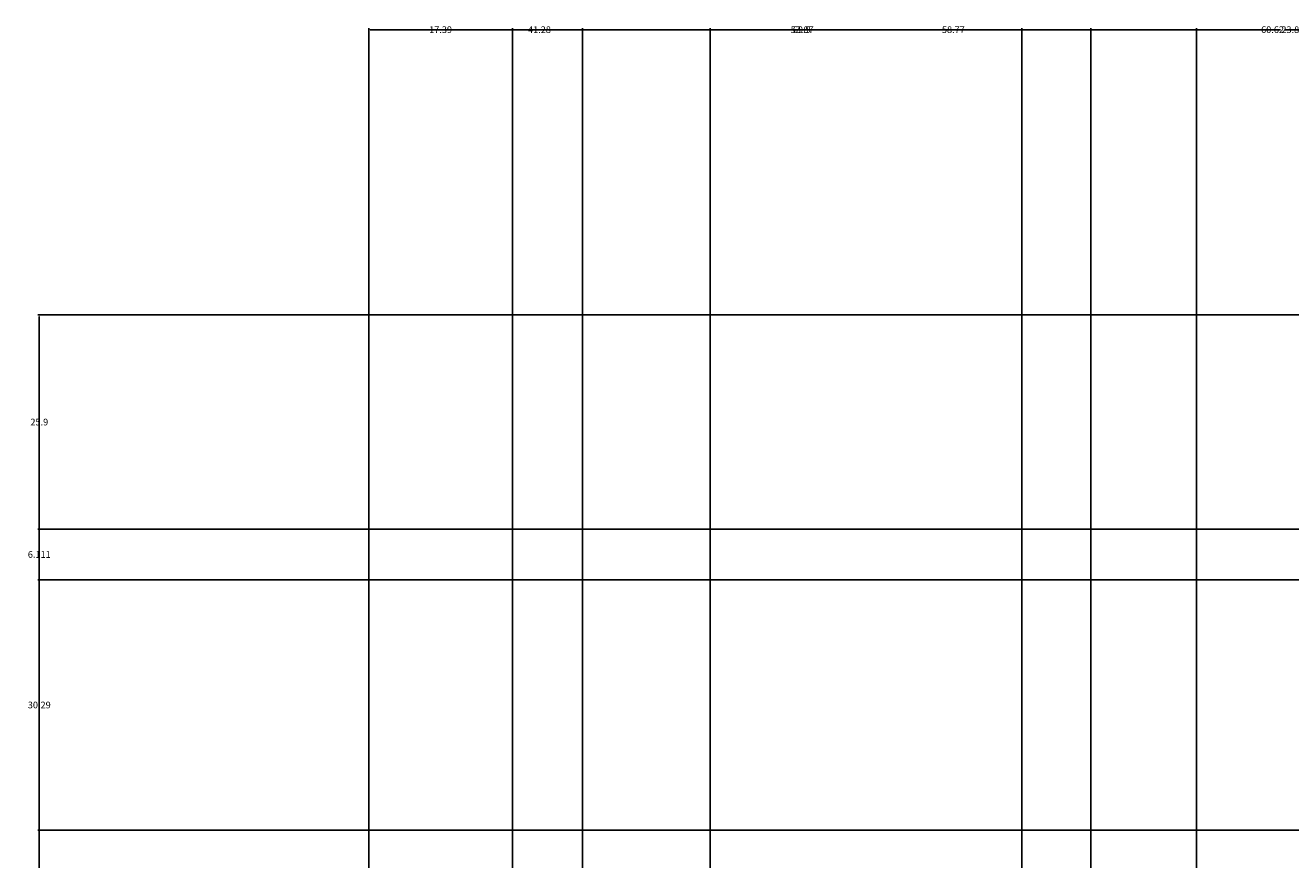
# Model space of a CAD drawing. Units: inches. Extents: x 36 to 594, y 79 to 831.
# Tile 22 of 30: x 36 to 189, y 730 to 831. Entities that reach past the tile are written whole.
import ezdxf

# ---------------------------------------------------------------- set-up
doc = ezdxf.new("R2010")
doc.units = ezdxf.units.IN
doc.header["$MEASUREMENT"] = 0
doc.layers.add('A-ANNO-DIMS', color=2, linetype='Continuous', lineweight=18)
doc.styles.get("Standard").update_dxf_attribs({"font": 'arial.ttf'})
doc.dimstyles.get("Standard").update_dxf_attribs({"dimtxt": 0.8125, "dimasz": 0.18, "dimexe": 0.18, "dimexo": 0.0625, "dimgap": 0.09, "dimtad": 0, "dimtih": 1, "dimtoh": 1, "dimdec": 4, "dimzin": 0, "dimdsep": 46, "dimlunit": 4, "dimtxsty": 'Standard', "dimcen": 0.09, "dimadec": 0, "dimazin": 0, "dimtfac": 1, "dimtdec": 4, "dimtofl": 0, "dimtmove": 0, "dimatfit": 3, "dimfxl": 1, "dimtolj": 1, "dimtzin": 0, "dimarcsym": 0})

# ---------------------------------------------------------------- blocks, each defined once
blk = doc.blocks.new('*D12')
at = {"layer": 'A-ANNO-DIMS', "color": 0, "lineweight": -2, "transparency": 16777216}
for p, q in [((77.48, 667.8), (77.48, 830.73)), ((77.66, 830.55), (96.64, 830.55)), ((118.58, 830.55), (99.6, 830.55)), ((118.76, 594.27), (118.76, 830.73))]:
    blk.add_line(p, q, dxfattribs=at)
at = {"layer": 'A-ANNO-DIMS', "color": 0, "transparency": 16777216}
for points in [[(77.66, 830.58), (77.66, 830.52), (77.48, 830.55)], [(118.58, 830.58), (118.58, 830.52), (118.76, 830.55)]]:
    blk.add_solid(points, dxfattribs=at)
at = {"layer": 'Defpoints', "color": 0, "transparency": 16777216}
for p in [(118.76, 830.55), (77.48, 667.73), (118.76, 594.21)]:
    blk.add_point(p, dxfattribs=at)
at = {"layer": 'A-ANNO-DIMS', "color": 0, "transparency": 16777216, "insert": (98.12, 830.55), "char_height": 0.812, "attachment_point": 5}
blk.add_mtext('\\A1;41.28', dxfattribs=at)
blk = doc.blocks.new('*D13')
at = {"layer": 'A-ANNO-DIMS', "color": 0, "lineweight": -2, "transparency": 16777216}
for p, q in [((118.76, 594.27), (118.76, 830.73)), ((118.94, 830.55), (146.68, 830.55)), ((177.34, 830.55), (149.6, 830.55)), ((177.52, 594.27), (177.52, 830.73))]:
    blk.add_line(p, q, dxfattribs=at)
at = {"layer": 'A-ANNO-DIMS', "color": 0, "transparency": 16777216}
for points in [[(118.94, 830.58), (118.94, 830.52), (118.76, 830.55)], [(177.34, 830.58), (177.34, 830.52), (177.52, 830.55)]]:
    blk.add_solid(points, dxfattribs=at)
at = {"layer": 'Defpoints', "color": 0, "transparency": 16777216}
for p in [(177.52, 830.55), (118.76, 594.21), (177.52, 594.21)]:
    blk.add_point(p, dxfattribs=at)
at = {"layer": 'A-ANNO-DIMS', "color": 0, "transparency": 16777216, "insert": (148.14, 830.55), "char_height": 0.812, "attachment_point": 5}
blk.add_mtext('\\A1;58.77', dxfattribs=at)
blk = doc.blocks.new('*D14')
at = {"layer": 'A-ANNO-DIMS', "color": 0, "lineweight": -2, "transparency": 16777216}
for p, q in [((177.52, 594.27), (177.52, 830.73)), ((177.7, 830.55), (187.69, 830.55)), ((201.24, 830.55), (191.25, 830.55)), ((201.42, 720.66), (201.42, 830.73))]:
    blk.add_line(p, q, dxfattribs=at)
at = {"layer": 'A-ANNO-DIMS', "color": 0, "transparency": 16777216}
for points in [[(177.7, 830.58), (177.7, 830.52), (177.52, 830.55)], [(201.24, 830.58), (201.24, 830.52), (201.42, 830.55)]]:
    blk.add_solid(points, dxfattribs=at)
at = {"layer": 'Defpoints', "color": 0, "transparency": 16777216}
for p in [(201.42, 830.55), (201.42, 720.59), (177.52, 594.21)]:
    blk.add_point(p, dxfattribs=at)
at = {"layer": 'A-ANNO-DIMS', "color": 0, "transparency": 16777216, "insert": (189.47, 830.55), "char_height": 0.812, "attachment_point": 5}
blk.add_mtext('\\A1;23.894', dxfattribs=at)
blk = doc.blocks.new('*D21')
at = {"layer": 'A-ANNO-DIMS', "color": 0, "lineweight": -2, "transparency": 16777216}
for p, q in [((77.48, 667.8), (77.48, 830.73)), ((77.66, 830.55), (84.75, 830.55)), ((94.69, 830.55), (87.59, 830.55)), ((94.87, 668.27), (94.87, 830.73))]:
    blk.add_line(p, q, dxfattribs=at)
at = {"layer": 'A-ANNO-DIMS', "color": 0, "transparency": 16777216}
for points in [[(77.66, 830.58), (77.66, 830.52), (77.48, 830.55)], [(94.69, 830.58), (94.69, 830.52), (94.87, 830.55)]]:
    blk.add_solid(points, dxfattribs=at)
at = {"layer": 'Defpoints', "color": 0, "transparency": 16777216}
for p in [(94.87, 830.55), (77.48, 667.73), (94.87, 668.21)]:
    blk.add_point(p, dxfattribs=at)
at = {"layer": 'A-ANNO-DIMS', "color": 0, "transparency": 16777216, "insert": (86.17, 830.55), "char_height": 0.812, "attachment_point": 5}
blk.add_mtext('\\A1;17.39', dxfattribs=at)
blk = doc.blocks.new('*D27')
at = {"layer": 'A-ANNO-DIMS', "color": 0, "lineweight": -2, "transparency": 16777216}
for p, q in [((94.87, 668.27), (94.87, 830.73)), ((95.05, 830.55), (128.67, 830.55)), ((164.59, 830.55), (130.96, 830.55)), ((164.77, 653.83), (164.77, 830.73))]:
    blk.add_line(p, q, dxfattribs=at)
at = {"layer": 'A-ANNO-DIMS', "color": 0, "transparency": 16777216}
for points in [[(95.05, 830.58), (95.05, 830.52), (94.87, 830.55)], [(164.59, 830.58), (164.59, 830.52), (164.77, 830.55)]]:
    blk.add_solid(points, dxfattribs=at)
at = {"layer": 'Defpoints', "color": 0, "transparency": 16777216}
for p in [(164.77, 830.55), (94.87, 668.21), (164.77, 653.76)]:
    blk.add_point(p, dxfattribs=at)
at = {"layer": 'A-ANNO-DIMS', "color": 0, "transparency": 16777216, "insert": (129.82, 830.55), "char_height": 0.812, "attachment_point": 5}
blk.add_mtext('\\A1;69.9', dxfattribs=at)
blk = doc.blocks.new('*D28')
at = {"layer": 'A-ANNO-DIMS', "color": 0, "lineweight": -2, "transparency": 16777216}
for p, q in [((269.3, 796.05), (37.49, 796.05)), ((37.67, 795.87), (37.67, 455.63)), ((37.67, 114.39), (37.67, 454.62)), ((94.8, 114.21), (37.49, 114.21))]:
    blk.add_line(p, q, dxfattribs=at)
at = {"layer": 'A-ANNO-DIMS', "color": 0, "transparency": 16777216}
for points in [[(37.64, 795.87), (37.7, 795.87), (37.67, 796.05)], [(37.64, 114.39), (37.7, 114.39), (37.67, 114.21)]]:
    blk.add_solid(points, dxfattribs=at)
at = {"layer": 'Defpoints', "color": 0, "transparency": 16777216}
for p in [(37.67, 796.05), (269.36, 796.05), (94.87, 114.21)]:
    blk.add_point(p, dxfattribs=at)
at = {"layer": 'A-ANNO-DIMS', "color": 0, "transparency": 16777216, "insert": (37.67, 455.13), "char_height": 0.812, "attachment_point": 5}
blk.add_mtext('\\A1;681.8', dxfattribs=at)
blk = doc.blocks.new('*D49')
at = {"layer": 'A-ANNO-DIMS', "color": 0, "lineweight": -2, "transparency": 16777216}
for p, q in [((209.97, 733.74), (37.49, 733.74)), ((37.67, 733.56), (37.67, 727.67)), ((37.67, 720.77), (37.67, 726.66)), ((201.36, 720.59), (37.49, 720.59))]:
    blk.add_line(p, q, dxfattribs=at)
at = {"layer": 'A-ANNO-DIMS', "color": 0, "transparency": 16777216}
for points in [[(37.64, 733.56), (37.7, 733.56), (37.67, 733.74)], [(37.64, 720.77), (37.7, 720.77), (37.67, 720.59)]]:
    blk.add_solid(points, dxfattribs=at)
at = {"layer": 'Defpoints', "color": 0, "transparency": 16777216}
for p in [(37.67, 733.74), (210.03, 733.74), (201.42, 720.59)]:
    blk.add_point(p, dxfattribs=at)
at = {"layer": 'A-ANNO-DIMS', "color": 0, "transparency": 16777216, "insert": (37.67, 727.17), "char_height": 0.812, "attachment_point": 5}
blk.add_mtext('\\A1;13.147', dxfattribs=at)
blk = doc.blocks.new('*D50')
at = {"layer": 'A-ANNO-DIMS', "color": 0, "lineweight": -2, "transparency": 16777216}
for p, q in [((260.51, 764.03), (37.49, 764.03)), ((37.67, 763.85), (37.67, 749.39)), ((37.67, 733.92), (37.67, 748.38)), ((209.97, 733.74), (37.49, 733.74))]:
    blk.add_line(p, q, dxfattribs=at)
at = {"layer": 'A-ANNO-DIMS', "color": 0, "transparency": 16777216}
for points in [[(37.64, 763.85), (37.7, 763.85), (37.67, 764.03)], [(37.64, 733.92), (37.7, 733.92), (37.67, 733.74)]]:
    blk.add_solid(points, dxfattribs=at)
at = {"layer": 'Defpoints', "color": 0, "transparency": 16777216}
for p in [(37.67, 764.03), (260.57, 764.03), (210.03, 733.74)]:
    blk.add_point(p, dxfattribs=at)
at = {"layer": 'A-ANNO-DIMS', "color": 0, "transparency": 16777216, "insert": (37.67, 748.89), "char_height": 0.812, "attachment_point": 5}
blk.add_mtext('\\A1;30.29', dxfattribs=at)
blk = doc.blocks.new('*D51')
at = {"layer": 'A-ANNO-DIMS', "color": 0, "lineweight": -2, "transparency": 16777216}
for p, q in [((260.51, 770.15), (37.49, 770.15)), ((37.67, 769.97), (37.67, 767.59)), ((37.67, 764.21), (37.67, 766.58)), ((260.51, 764.03), (37.49, 764.03))]:
    blk.add_line(p, q, dxfattribs=at)
at = {"layer": 'A-ANNO-DIMS', "color": 0, "transparency": 16777216}
for points in [[(37.64, 769.97), (37.7, 769.97), (37.67, 770.15)], [(37.64, 764.21), (37.7, 764.21), (37.67, 764.03)]]:
    blk.add_solid(points, dxfattribs=at)
at = {"layer": 'Defpoints', "color": 0, "transparency": 16777216}
for p in [(37.67, 770.15), (260.57, 770.15), (260.57, 764.03)]:
    blk.add_point(p, dxfattribs=at)
at = {"layer": 'A-ANNO-DIMS', "color": 0, "transparency": 16777216, "insert": (37.67, 767.09), "char_height": 0.812, "attachment_point": 5}
blk.add_mtext('\\A1;6.111', dxfattribs=at)
blk = doc.blocks.new('*D52')
at = {"layer": 'A-ANNO-DIMS', "color": 0, "lineweight": -2, "transparency": 16777216}
for p, q in [((269.3, 796.05), (37.49, 796.05)), ((37.67, 795.87), (37.67, 783.6)), ((37.67, 770.33), (37.67, 782.59)), ((260.51, 770.15), (37.49, 770.15))]:
    blk.add_line(p, q, dxfattribs=at)
at = {"layer": 'A-ANNO-DIMS', "color": 0, "transparency": 16777216}
for points in [[(37.64, 795.87), (37.7, 795.87), (37.67, 796.05)], [(37.64, 770.33), (37.7, 770.33), (37.67, 770.15)]]:
    blk.add_solid(points, dxfattribs=at)
at = {"layer": 'Defpoints', "color": 0, "transparency": 16777216}
for p in [(37.67, 796.05), (269.36, 796.05), (260.57, 770.15)]:
    blk.add_point(p, dxfattribs=at)
at = {"layer": 'A-ANNO-DIMS', "color": 0, "transparency": 16777216, "insert": (37.67, 783.1), "char_height": 0.812, "attachment_point": 5}
blk.add_mtext('\\A1;25.9', dxfattribs=at)
blk = doc.blocks.new('*D60')
at = {"layer": 'A-ANNO-DIMS', "color": 0, "lineweight": -2, "transparency": 16777216}
for p, q in [((103.34, 286.24), (103.34, 830.73)), ((103.52, 830.55), (128.41, 830.55)), ((156.23, 830.55), (131.33, 830.55)), ((156.41, 264.68), (156.41, 830.73))]:
    blk.add_line(p, q, dxfattribs=at)
at = {"layer": 'A-ANNO-DIMS', "color": 0, "transparency": 16777216}
for points in [[(103.52, 830.58), (103.52, 830.52), (103.34, 830.55)], [(156.23, 830.58), (156.23, 830.52), (156.41, 830.55)]]:
    blk.add_solid(points, dxfattribs=at)
at = {"layer": 'Defpoints', "color": 0, "transparency": 16777216}
for p in [(156.41, 830.55), (103.34, 286.18), (156.41, 264.62)]:
    blk.add_point(p, dxfattribs=at)
at = {"layer": 'A-ANNO-DIMS', "color": 0, "transparency": 16777216, "insert": (129.87, 830.55), "char_height": 0.812, "attachment_point": 5}
blk.add_mtext('\\A1;53.07', dxfattribs=at)
blk = doc.blocks.new('*D61')
at = {"layer": 'A-ANNO-DIMS', "color": 0, "lineweight": -2, "transparency": 16777216}
for p, q in [((156.41, 264.68), (156.41, 830.73)), ((156.59, 830.55), (185.26, 830.55)), ((216.85, 830.55), (188.18, 830.55)), ((217.03, 286.24), (217.03, 830.73))]:
    blk.add_line(p, q, dxfattribs=at)
at = {"layer": 'A-ANNO-DIMS', "color": 0, "transparency": 16777216}
for points in [[(156.59, 830.58), (156.59, 830.52), (156.41, 830.55)], [(216.85, 830.58), (216.85, 830.52), (217.03, 830.55)]]:
    blk.add_solid(points, dxfattribs=at)
at = {"layer": 'Defpoints', "color": 0, "transparency": 16777216}
for p in [(217.03, 830.55), (217.03, 286.18), (156.41, 264.62)]:
    blk.add_point(p, dxfattribs=at)
at = {"layer": 'A-ANNO-DIMS', "color": 0, "transparency": 16777216, "insert": (186.72, 830.55), "char_height": 0.812, "attachment_point": 5}
blk.add_mtext('\\A1;60.62', dxfattribs=at)

msp = doc.modelspace()

# ---------------------------------------------------------------- dimensions: what is measured, and where the dimension line sits
at = {"layer": 'A-ANNO-DIMS'}
for base, p1, p2, override, picture, middle in [((118.7598, 830.5465), (77.477, 667.7335), (118.7598, 594.2124), {"dimdec": 2, "dimlfac": 1, "dimrnd": 0, "dimzin": 0, "dimdsep": 46, "dimlunit": 2}, '*D12', (98.1184, 830.5465)), ((94.8658, 830.5465), (77.477, 667.7335), (94.8658, 668.2124), {"dimdec": 2, "dimlfac": 1, "dimrnd": 0, "dimzin": 0, "dimdsep": 46, "dimlunit": 2}, '*D21', (86.1714, 830.5465)), ((164.7665, 830.5465), (94.8658, 668.2124), (164.7665, 653.7648), {"dimdec": 1, "dimlfac": 1, "dimrnd": 0, "dimzin": 0, "dimdsep": 46, "dimlunit": 2}, '*D27', (129.8161, 830.5465)), ((156.4069, 830.5465), (103.3368, 286.1802), (156.4069, 264.6224), {"dimdec": 2, "dimlfac": 1, "dimrnd": 0, "dimzin": 0, "dimdsep": 46, "dimlunit": 2}, '*D60', (129.8718, 830.5465)), ((177.525, 830.5465), (118.7598, 594.2124), (177.525, 594.2124), {"dimdec": 2, "dimlfac": 1, "dimrnd": 0, "dimzin": 0, "dimdsep": 46, "dimlunit": 2}, '*D13', (148.1424, 830.5465)), ((217.0273, 830.5465), (156.4069, 264.6224), (217.0273, 286.1802), {"dimdec": 2, "dimlfac": 1, "dimrnd": 0, "dimzin": 0, "dimdsep": 46, "dimlunit": 2}, '*D61', (186.7171, 830.5465)), ((201.4189, 830.5465), (177.525, 594.2124), (201.4189, 720.595), {"dimdec": 3, "dimlfac": 1, "dimrnd": 0, "dimzin": 0, "dimdsep": 46, "dimlunit": 2}, '*D14', (189.4719, 830.5465))]:
    dim = msp.add_linear_dim(base=base, p1=p1, p2=p2, dimstyle='Standard', override=override, dxfattribs=at)
    dim.commit()
    dim.dimension.update_dxf_attribs({"geometry": picture, "text_midpoint": middle})
for base, p1, p2, override, picture, middle in [((37.6733, 796.0465), (94.8658, 114.2124), (269.3592, 796.0465), {"dimdec": 1, "dimlfac": 1, "dimrnd": 0, "dimzin": 0, "dimdsep": 46, "dimlunit": 2}, '*D28', (37.6733, 455.1294)), ((37.6733, 796.0465), (260.5727, 770.1455), (269.3592, 796.0465), {"dimdec": 1, "dimlfac": 1, "dimrnd": 0, "dimzin": 0, "dimdsep": 46, "dimlunit": 2}, '*D52', (37.6733, 783.096)), ((37.6733, 770.1455), (260.5727, 764.0341), (260.5727, 770.1455), {"dimdec": 3, "dimlfac": 1, "dimrnd": 0, "dimzin": 0, "dimdsep": 46, "dimlunit": 2}, '*D51', (37.6733, 767.0898)), ((37.6733, 764.0341), (210.028, 733.7417), (260.5727, 764.0341), {"dimdec": 2, "dimlfac": 1, "dimrnd": 0, "dimzin": 0, "dimdsep": 46, "dimlunit": 2}, '*D50', (37.6733, 748.8879)), ((37.6733, 733.7417), (201.4189, 720.595), (210.028, 733.7417), {"dimdec": 3, "dimlfac": 1, "dimrnd": 0, "dimzin": 0, "dimdsep": 46, "dimlunit": 2}, '*D49', (37.6733, 727.1683))]:
    dim = msp.add_linear_dim(base=base, p1=p1, p2=p2, angle=90, dimstyle='Standard', override=override, dxfattribs=at)
    dim.commit()
    dim.dimension.update_dxf_attribs({"geometry": picture, "text_midpoint": middle})

doc.saveas('drawing.dxf')
